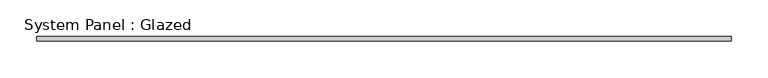
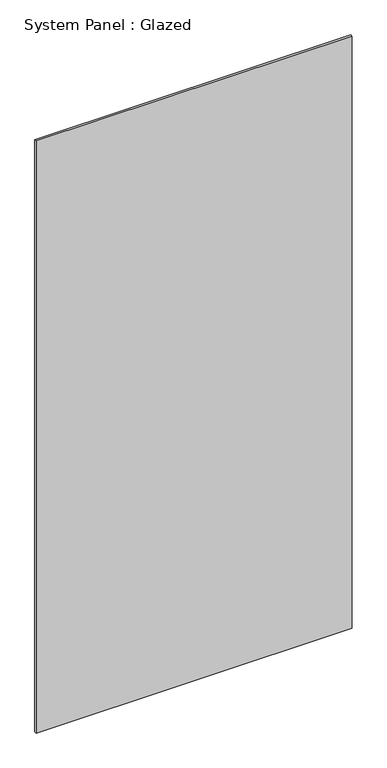
"""IFC4 building model written with IfcOpenShell, lengths in millimetres: plate geometry, System Panel : Glazed."""

from ifc_helpers import new_model, si_unit, origin, origin_with_axes, place, context, project, spatial, polyline, outline, extrude, source, transform, mapped, element, save


def system_panel_glazed_fc828323(model_context):
    return source(origin(), model_context, "Body", "SweptSolid", [
        extrude(outline(polyline([(470.8333334, 34.0), (-470.8333334, 34.0), (-470.8333334, 40.0), (470.8333334, 40.0), (470.8333334, 34.0)])), origin_with_axes(), (0.0, 0.0, 1.0), 1865.4113705),
    ])


if __name__ == "__main__":
    model = new_model("IFC4")
    model_context = context("Model", 3, world=origin())
    ifc_project = project(units=[si_unit("LENGTHUNIT", "METRE", prefix="MILLI")], contexts=[model_context])
    site = spatial("IfcSite", under=ifc_project)
    building = spatial("IfcBuilding", under=site)
    placement = place(None, origin())
    system_panel_glazed_shape = system_panel_glazed_fc828323(model_context)
    element("IfcPlate", 1, ObjectType="System Panel : Glazed", at=placement, inside=building, context=model_context, shape_type="MappedRepresentation", body=[
        mapped(system_panel_glazed_shape, transform((0.0, 0.0, 0.0), x_axis=(1.0, 0.0, 0.0), y_axis=(0.0, 1.0, 0.0), z_axis=(0.0, 0.0, 1.0))),
    ])
    save(model, "model.ifc")

# Revit data of these elements
# Type "System Panel : Glazed"
#   Construction Type Id = "GSP4R"
#   Analytic Construction = "1/8 in Pilkington single glazing"
#   Visual Light Transmittance = 0.9
#   Solar Heat Gain Coefficient = 0.86
#   Heat Transfer Coefficient (U) = 6.7069 W/(m²·K)
#   Define Thermal Properties by = 1
# Element 1 (IfcPlate, "System Panel : Glazed")
#   Materials on its faces: "Default New Material(6)"
# Materials
#   "Default New Material(6)": class "Generic", colour RGB 191 25 25, transparency 0.9, Cost = 0
